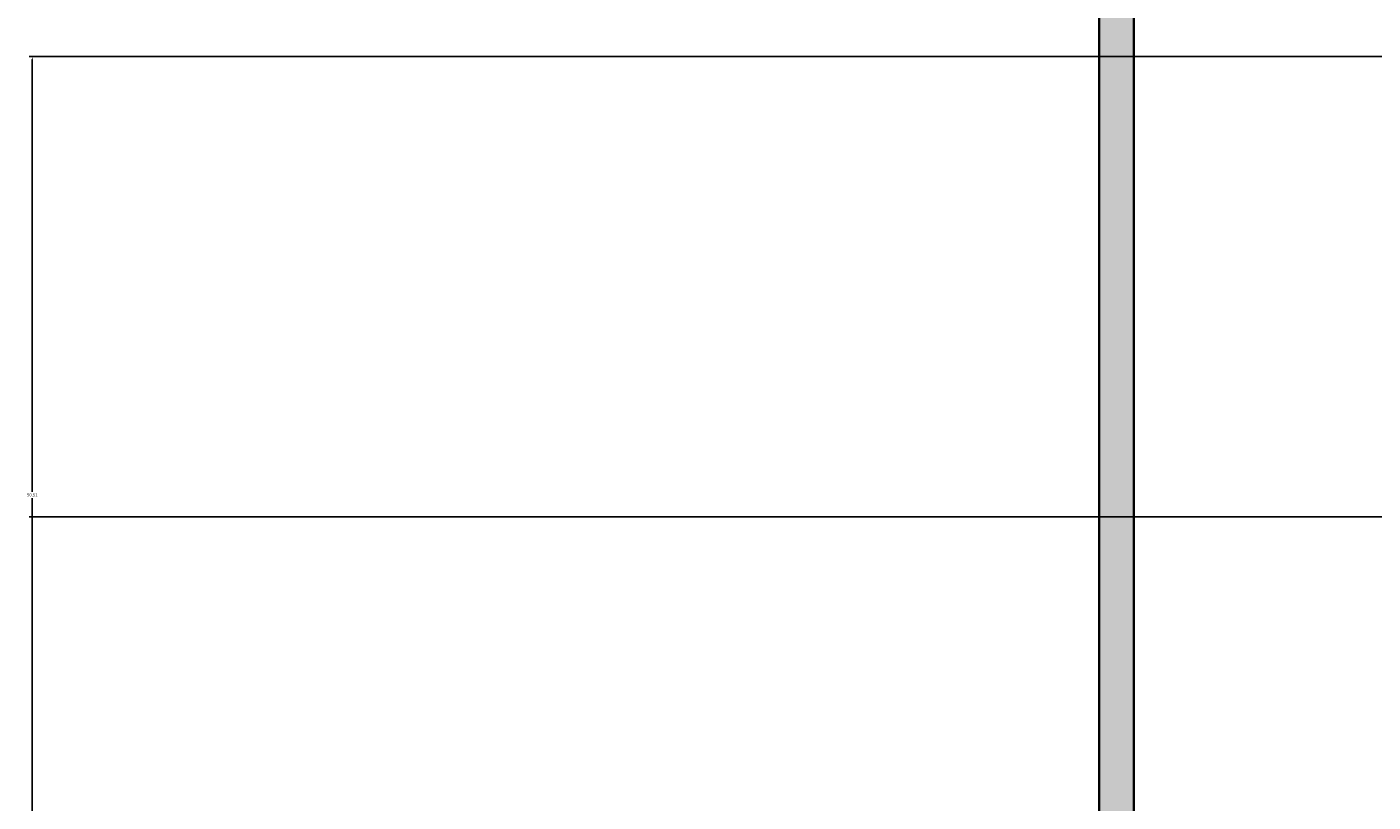
# Model space of a CAD drawing. Units: inches. Extents: x 1998 to 2588, y 1139 to 1977.
# Tile 6 of 134: x 1998 to 2075, y 1620 to 1665. Entities that reach past the tile are written whole.
import ezdxf

# ---------------------------------------------------------------- set-up
doc = ezdxf.new("R2010")
doc.units = ezdxf.units.IN
for name, color, linetype, lineweight in [('A-ANNO-DIMS', 2, 'Continuous', 18), ('A-WALL-PATT', 252, 'Continuous', 13), ('WALL', 200, 'Continuous', 35)]:
    doc.layers.add(name, color=color, linetype=linetype, lineweight=lineweight)
doc.styles.get("Standard").update_dxf_attribs({"font": 'arial.ttf'})
doc.dimstyles.get("Standard").update_dxf_attribs({"dimtxt": 0.18, "dimasz": 0.18, "dimexe": 0.18, "dimexo": 0.0625, "dimgap": 0.09, "dimtad": 0, "dimtih": 1, "dimtoh": 1, "dimdec": 4, "dimzin": 0, "dimdsep": 46, "dimtxsty": 'Standard', "dimcen": 0.09, "dimadec": 0, "dimazin": 0, "dimtfac": 1, "dimtdec": 4, "dimtofl": 0, "dimtmove": 0, "dimatfit": 3, "dimfxl": 1, "dimtolj": 1, "dimtzin": 0, "dimarcsym": 0})

# ---------------------------------------------------------------- blocks, each defined once
blk = doc.blocks.new('*D30')
at = {"layer": 'A-ANNO-DIMS', "color": 0, "lineweight": -2, "transparency": 16777216}
for p, q in [((2407.91, 1636.732), (1997.843, 1636.732)), ((1998.023, 1636.552), (1998.023, 1615.913)), ((1998.023, 1594.912), (1998.023, 1615.552)), ((2407.91, 1594.732), (1997.843, 1594.732))]:
    blk.add_line(p, q, dxfattribs=at)
at = {"layer": 'A-ANNO-DIMS', "color": 0, "transparency": 16777216}
for points in [[(1997.993, 1636.552), (1998.053, 1636.552), (1998.023, 1636.732)], [(1997.993, 1594.912), (1998.053, 1594.912), (1998.023, 1594.732)]]:
    blk.add_solid(points, dxfattribs=at)
at = {"layer": 'Defpoints', "color": 0, "transparency": 16777216}
for p in [(1998.023, 1636.732), (2407.973, 1636.732), (2407.973, 1594.732)]:
    blk.add_point(p, dxfattribs=at)
at = {"layer": 'A-ANNO-DIMS', "color": 0, "transparency": 16777216, "insert": (1998.023, 1615.732), "char_height": 0.18, "attachment_point": 5}
blk.add_mtext('\\A1;42', dxfattribs=at)
blk = doc.blocks.new('*D38')
at = {"layer": 'A-ANNO-DIMS', "color": 0, "lineweight": -2, "transparency": 16777216}
for p, q in [((2197.387, 1663.247), (1997.843, 1663.247)), ((1998.023, 1663.067), (1998.023, 1638.171)), ((1998.023, 1612.912), (1998.023, 1637.808)), ((2197.387, 1612.732), (1997.843, 1612.732))]:
    blk.add_line(p, q, dxfattribs=at)
at = {"layer": 'A-ANNO-DIMS', "color": 0, "transparency": 16777216}
for points in [[(1997.993, 1663.067), (1998.053, 1663.067), (1998.023, 1663.247)], [(1997.993, 1612.912), (1998.053, 1612.912), (1998.023, 1612.732)]]:
    blk.add_solid(points, dxfattribs=at)
at = {"layer": 'Defpoints', "color": 0, "transparency": 16777216}
for p in [(1998.023, 1663.247), (2197.45, 1663.247), (2197.45, 1612.732)]:
    blk.add_point(p, dxfattribs=at)
at = {"layer": 'A-ANNO-DIMS', "color": 0, "transparency": 16777216, "insert": (1998.023, 1637.99), "char_height": 0.18, "attachment_point": 5}
blk.add_mtext('\\A1;50.51', dxfattribs=at)

msp = doc.modelspace()

# ---------------------------------------------------------------- hatches: boundary and pattern name
at = {"layer": 'A-WALL-PATT'}
h = msp.add_hatch(color=256, dxfattribs=at)
h.dxf.hatch_style = 1
h.paths.add_polyline_path([(2227.4729, 1911.2324), (2222.9729, 1911.2324), (2222.9729, 1888.7324), (2227.4729, 1888.7324)])
h.paths.add_polyline_path([(2236.4493, 1870.3636), (2236.4493, 1875.2324), (2234.4125, 1875.2324), (2234.4125, 1868.3278), (2227.4729, 1868.3278), (2227.4729, 1866.2324), (2236.4493, 1866.2324)])
h.paths.add_polyline_path([(2330.0332, 1875.2324), (2263.9907, 1875.2324), (2263.9907, 1866.2324), (2330.0332, 1866.2324)])
h.paths.add_polyline_path([(2345.9729, 1906.7324), (2393.9729, 1906.7324), (2393.9729, 1882.7324), (2345.9729, 1882.7324), (2345.9729, 1878.2324), (2393.9729, 1878.2324), (2398.4729, 1878.2324), (2398.4729, 1882.7324), (2398.4729, 1911.2324), (2345.9729, 1911.2324), (2341.4729, 1911.2324), (2341.4729, 1866.2324), (2341.4729, 1790.0412), (2345.9729, 1790.0412), (2345.9729, 1875.2324)])
h.paths.add_polyline_path([(2398.4729, 1878.2324), (2393.9729, 1878.2324), (2393.9729, 1798.2324), (2393.9729, 1793.7324), (2398.4729, 1793.7324)], flags=17)
h.paths.add_polyline_path([(2393.9729, 1798.2324), (2375.7311, 1798.2324, -0.005968), (2375.7384, 1797.6146), (2375.7384, 1793.7324), (2393.9729, 1793.7324)], flags=17)
h.paths.add_polyline_path([(2349.8569, 1797.6146), (2349.8569, 1798.2324), (2345.9729, 1798.2324), (2345.9729, 1793.7324), (2349.8569, 1793.7324)], flags=17)
h.paths.add_polyline_path([(2398.4729, 1793.7324), (2393.9729, 1793.7324), (2393.9729, 1790.0412), (2398.4729, 1790.0412)], flags=17)
h.paths.add_polyline_path([(2527.4729, 1882.7324), (2507.8006, 1882.7324), (2507.8006, 1878.2324), (2518.4729, 1878.2324), (2518.4729, 1759.7324), (2510.9729, 1759.7324), (2510.9729, 1755.2324), (2527.4729, 1755.2324)])
h.paths.add_polyline_path([(2487.396, 1882.7324), (2398.4729, 1882.7324), (2398.4729, 1878.2324), (2487.396, 1878.2324)])
h.paths.add_polyline_path([(2490.5682, 1759.7324), (2345.9729, 1759.7324), (2345.9729, 1755.2324), (2490.5682, 1755.2324)])
h.paths.add_polyline_path([(2398.4729, 1760.5844), (2398.3914, 1760.5844), (2393.9729, 1760.5844), (2393.9729, 1759.7324), (2398.4729, 1759.7324)])
h.paths.add_polyline_path([(2334.5332, 1759.7324), (2234.4125, 1759.7324), (2234.4125, 1755.2324), (2334.5332, 1755.2324)])
h.paths.add_polyline_path([(2345.9729, 1760.5844), (2341.5543, 1760.5844), (2341.4729, 1760.5844), (2341.4729, 1759.7324), (2345.9729, 1759.7324)])
h.paths.add_polyline_path([(2222.9729, 1759.7324), (2221.7204, 1759.7324), (2221.7204, 1755.2324), (2222.9729, 1755.2324)])
h.paths.add_polyline_path([(2061.4729, 1702.7324), (2059.4729, 1702.7324), (2059.4729, 1584.2324), (2061.4729, 1584.2324)])
h.paths.add_polyline_path([(2061.4729, 1584.2324), (2059.4729, 1584.2324), (2059.4729, 1470.2324), (2061.4729, 1470.2324)])
h.paths.add_polyline_path([(2510.9729, 1469.2927), (2501.9729, 1469.2927), (2501.9729, 1369.172), (2510.9729, 1369.172)])
h.paths.add_polyline_path([(2227.4729, 1369.7324), (2227.4729, 1417.7324), (2221.4126, 1417.7324), (2221.4126, 1413.2324), (2222.9729, 1413.2324), (2222.9729, 1293.2324), (2222.9729, 1285.137), (2227.4729, 1285.137)])

# ---------------------------------------------------------------- linework, layer by layer
at = {"layer": 'WALL'}
for p, q in [((2061.4729, 1473.2749), (2061.4729, 1705.7749)), ((2059.4729, 1470.2324), (2059.4729, 1702.7324))]:
    msp.add_line(p, q, dxfattribs=at)
msp.add_lwpolyline([(2059.4729, 1584.2324), (2061.4729, 1584.2324), (2061.4729, 1702.7324), (2059.4729, 1702.7324)], close=True, dxfattribs=at)

# ---------------------------------------------------------------- dimensions: what is measured, and where the dimension line sits
at = {"layer": 'A-ANNO-DIMS'}
for base, p1, p2, override, picture, middle in [((1998.0229, 1663.2466), (2197.4499, 1612.7324), (2197.4499, 1663.2466), {"dimdec": 2, "dimlfac": 1, "dimrnd": 0, "dimzin": 0, "dimdsep": 46, "dimlunit": 2}, '*D38', (1998.0229, 1637.9895)), ((1998.0229, 1636.7324), (2407.9729, 1594.7324), (2407.9729, 1636.7324), {"dimdec": 0, "dimlfac": 1, "dimrnd": 0, "dimzin": 0, "dimdsep": 46, "dimlunit": 2}, '*D30', (1998.0229, 1615.7324))]:
    dim = msp.add_linear_dim(base=base, p1=p1, p2=p2, angle=90, dimstyle='Standard', override=override, dxfattribs=at)
    dim.commit()
    dim.dimension.update_dxf_attribs({"geometry": picture, "text_midpoint": middle})

doc.saveas('drawing.dxf')
